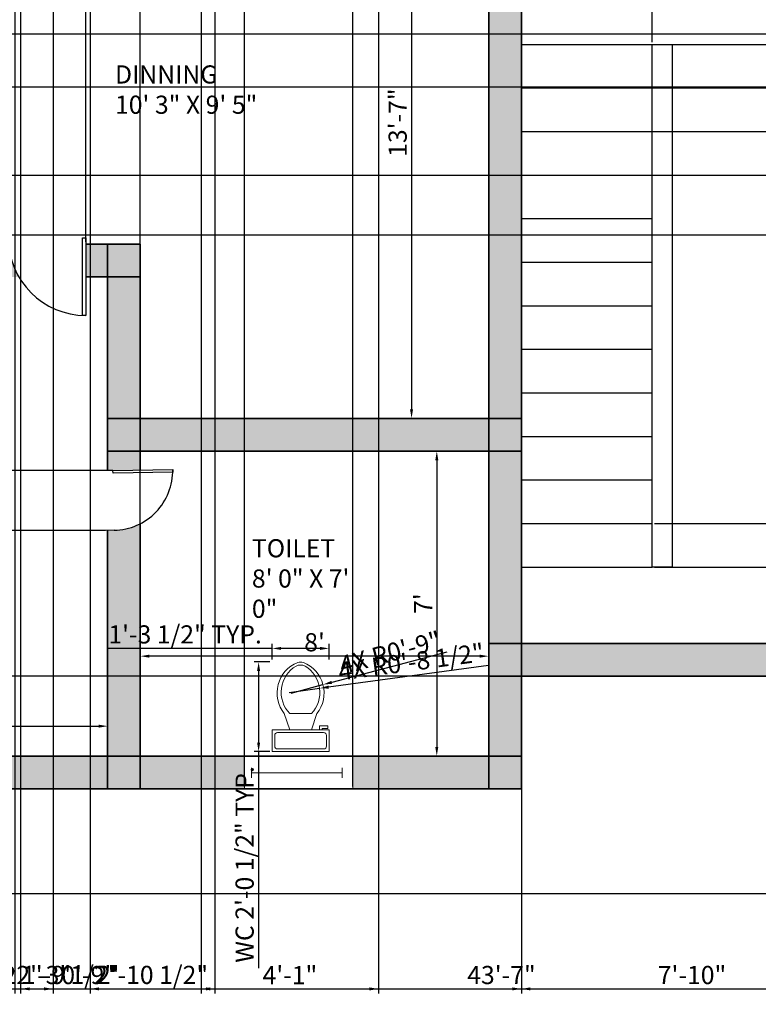
# Model space of a CAD drawing. Units: millimetres. Extents: x 2803 to 3393, y 965 to 1464.
# Tile 2 of 6: x 2968 to 3172, y 965 to 1236. Entities that reach past the tile are written whole.
import ezdxf

# ---------------------------------------------------------------- set-up
doc = ezdxf.new("R2010")
doc.units = ezdxf.units.MM
for name, color, linetype, lineweight in [('A-ANNO-DIMS', 150, 'Continuous', 18), ('A-AREA-IDEN', 200, 'Continuous', 25), ('A-FLOR-FIXT', 70, 'Continuous', 18), ('A-WALL-PATT', 2, 'Continuous', 13), ('doors', 10, 'Continuous', 25), ('staircase', 130, 'Continuous', 25), ('walls', 2, 'Continuous', 35), ('windows', 30, 'Continuous', 20)]:
    doc.layers.add(name, color=color, linetype=linetype, lineweight=lineweight)
doc.styles.get("Standard").update_dxf_attribs({"font": 'arial.ttf'})
doc.dimstyles.new('ISO-25', dxfattribs={"dimtxt": 5, "dimasz": 2.5, "dimexe": 1.25, "dimexo": 0.625, "dimtad": 1, "dimdec": 0, "dimlunit": 3, "dimtxsty": 'Standard', "dimcen": 2.5, "dimadec": 0, "dimazin": 0, "dimtfac": 1, "dimtdec": 0, "dimtmove": 0, "dimatfit": 3, "dimfxl": 1, "dimarcsym": 0})

# ---------------------------------------------------------------- blocks, each defined once
blk = doc.blocks.new('*U2')
for p, q in [((0, 0), (0, -6)), ((40, 0), (40, -6))]:
    blk.add_line(p, q)
blk.add_lwpolyline([(0, 0), (0, 40), (1.75, 40), (1.75, 0)], close=True)
blk.add_arc((0, 0), 40, 0, 90)
blk = doc.blocks.new('*U6')
for p, q in [((0, 4), (0, 0)), ((36, 4), (36, 0)), ((0, 2), (36, 2))]:
    blk.add_line(p, q)
blk = doc.blocks.new('Toilet - top')
for p, q in [((9.5, -6), (9.5, -2)), ((-10, -8.5), (-8, -8.5)), ((-10, -9.5), (-10, -8.5)), ((-7, -9.5), (-10, -9.5)), ((-8, -8.5), (-8, -8)), ((-7, -8), (-7, -9.5)), ((-4, -8), (-6, -14)), ((4, -8), (6, -14)), ((4, -14), (-4, -14))]:
    blk.add_line(p, q)
blk.add_lwpolyline([(10.5, -8), (10.5, 0), (-10.5, 0), (-10.5, -8)], close=True)
for points in [[(-9.5, -2), (-9.5, -6)], [(8.5, -1), (-8.5, -1)], [(-8.5, -7), (8.5, -7)]]:
    blk.add_lwpolyline(points)
for centre, radius, start, end in [((-8.62, -1.88), 0.884, 81.8699, 188.1301), ((8.62, -1.88), 0.884, 351.8699, 98.1301), ((-8.62, -6.12), 0.884, 171.8699, 278.1301), ((8.62, -6.12), 0.884, 261.8699, 8.1301), ((3.52, -21.58), 12.17, 141.4691, 247.9714), ((4.2, -21.82), 11.33, 136.3677, 238.9468), ((-3.52, -21.58), 12.17, 292.0284, 38.5307), ((-4.2, -21.82), 11.33, 301.053, 43.6321), ((0, -27.88), 4, 245.7318, 294.2682), ((0, -29), 4, 254.8605, 285.1395)]:
    blk.add_arc(centre, radius, start, end)
blk = doc.blocks.new('*D19')
at = {"layer": 'A-ANNO-DIMS', "color": 0, "lineweight": -2, "transparency": 16777216}
for p, q in [((3077.03, 1289.56), (3077.66, 1289.56)), ((3076.41, 1287.06), (3076.41, 1129.06)), ((3077.03, 1126.56), (3077.66, 1126.56))]:
    blk.add_line(p, q, dxfattribs=at)
at = {"layer": 'A-ANNO-DIMS', "color": 0, "transparency": 16777216}
for points in [[(3075.99, 1287.06), (3076.82, 1287.06), (3076.41, 1289.56)], [(3075.99, 1129.06), (3076.82, 1129.06), (3076.41, 1126.56)]]:
    blk.add_solid(points, dxfattribs=at)
at = {"layer": 'Defpoints', "color": 0, "transparency": 16777216}
for p in [(3076.41, 1289.56), (3076.41, 1126.56), (3076.41, 1126.56)]:
    blk.add_point(p, dxfattribs=at)
at = {"layer": 'A-ANNO-DIMS', "color": 0, "transparency": 16777216, "insert": (3073.23, 1208.06), "char_height": 5, "attachment_point": 5, "rotation": 90}
blk.add_mtext('13\'-7"', dxfattribs=at)
blk = doc.blocks.new('*D25')
at = {"layer": 'A-ANNO-DIMS', "color": 0, "lineweight": -2, "transparency": 16777216}
for p, q in [((2848.68, 1045.62), (2848.68, 1040.53)), ((2992.68, 1045.62), (2992.68, 1040.53)), ((2851.18, 1041.78), (2990.18, 1041.78))]:
    blk.add_line(p, q, dxfattribs=at)
at = {"layer": 'A-ANNO-DIMS', "color": 0, "transparency": 16777216}
for points in [[(2851.18, 1042.2), (2851.18, 1041.37), (2848.68, 1041.78)], [(2990.18, 1042.2), (2990.18, 1041.37), (2992.68, 1041.78)]]:
    blk.add_solid(points, dxfattribs=at)
at = {"layer": 'Defpoints', "color": 0, "transparency": 16777216}
for p in [(2848.68, 1046.25), (2992.68, 1046.25), (2992.68, 1041.78)]:
    blk.add_point(p, dxfattribs=at)
at = {"layer": 'A-ANNO-DIMS', "color": 0, "transparency": 16777216, "insert": (2920.68, 1044.92), "char_height": 5, "attachment_point": 5}
blk.add_mtext("12'", dxfattribs=at)
blk = doc.blocks.new('*D26')
at = {"layer": 'A-ANNO-DIMS', "color": 0, "lineweight": -2, "transparency": 16777216}
for p, q in [((3085.22, 1117.56), (3082.11, 1117.56)), ((3083.36, 1115.06), (3083.36, 1036.06)), ((3085.22, 1033.56), (3082.11, 1033.56))]:
    blk.add_line(p, q, dxfattribs=at)
at = {"layer": 'A-ANNO-DIMS', "color": 0, "transparency": 16777216}
for points in [[(3082.95, 1115.06), (3083.78, 1115.06), (3083.36, 1117.56)], [(3082.95, 1036.06), (3083.78, 1036.06), (3083.36, 1033.56)]]:
    blk.add_solid(points, dxfattribs=at)
at = {"layer": 'Defpoints', "color": 0, "transparency": 16777216}
for p in [(3085.85, 1117.56), (3083.36, 1033.56), (3085.85, 1033.56)]:
    blk.add_point(p, dxfattribs=at)
at = {"layer": 'A-ANNO-DIMS', "color": 0, "transparency": 16777216, "insert": (3080.24, 1075.56), "char_height": 5, "attachment_point": 5, "rotation": 90}
blk.add_mtext("7'", dxfattribs=at)
blk = doc.blocks.new('*D27')
at = {"layer": 'A-ANNO-DIMS', "color": 0, "lineweight": -2, "transparency": 16777216}
for p, q in [((3001.68, 1063.94), (3001.68, 1059.82)), ((3097.68, 1063.94), (3097.68, 1059.82)), ((3095.18, 1061.07), (3004.18, 1061.07))]:
    blk.add_line(p, q, dxfattribs=at)
at = {"layer": 'A-ANNO-DIMS', "color": 0, "transparency": 16777216}
for points in [[(3004.18, 1061.49), (3004.18, 1060.65), (3001.68, 1061.07)], [(3095.18, 1061.49), (3095.18, 1060.65), (3097.68, 1061.07)]]:
    blk.add_solid(points, dxfattribs=at)
at = {"layer": 'Defpoints', "color": 0, "transparency": 16777216}
for p in [(3001.68, 1064.56), (3097.68, 1064.56), (3001.68, 1061.07)]:
    blk.add_point(p, dxfattribs=at)
at = {"layer": 'A-ANNO-DIMS', "color": 0, "transparency": 16777216, "insert": (3049.68, 1064.25), "char_height": 5, "attachment_point": 5}
blk.add_mtext("8'", dxfattribs=at)
blk = doc.blocks.new('*D31')
at = {"layer": 'A-ANNO-DIMS', "color": 0, "lineweight": -2, "transparency": 16777216}
for p, q in [((3037.35, 1059.49), (3033.02, 1059.49)), ((3034.27, 1056.99), (3034.27, 1037.26)), ((3037.35, 1034.76), (3033.02, 1034.76)), ((3034.27, 1034.76), (3034.27, 975.1))]:
    blk.add_line(p, q, dxfattribs=at)
at = {"layer": 'A-ANNO-DIMS', "color": 0, "transparency": 16777216}
for points in [[(3033.85, 1056.99), (3034.68, 1056.99), (3034.27, 1059.49)], [(3033.85, 1037.26), (3034.68, 1037.26), (3034.27, 1034.76)]]:
    blk.add_solid(points, dxfattribs=at)
at = {"layer": 'Defpoints', "color": 0, "transparency": 16777216}
for p in [(3037.98, 1059.49), (3034.27, 1034.76), (3037.98, 1034.76)]:
    blk.add_point(p, dxfattribs=at)
at = {"layer": 'A-ANNO-DIMS', "color": 0, "transparency": 16777216, "insert": (3031.06, 1003.68), "char_height": 5, "attachment_point": 5, "rotation": 90}
blk.add_mtext('WC 2\'-0 1/2" TYP.', dxfattribs=at)
blk = doc.blocks.new('*D32')
at = {"layer": 'A-ANNO-DIMS', "color": 0, "lineweight": -2, "transparency": 16777216}
for p, q in [((3037.98, 1060.12), (3037.98, 1064.45)), ((3053.69, 1060.12), (3053.69, 1064.45)), ((3037.98, 1063.2), (2992.57, 1063.2)), ((3051.19, 1063.2), (3040.48, 1063.2))]:
    blk.add_line(p, q, dxfattribs=at)
at = {"layer": 'A-ANNO-DIMS', "color": 0, "transparency": 16777216}
for points in [[(3040.48, 1063.62), (3040.48, 1062.79), (3037.98, 1063.2)], [(3051.19, 1063.62), (3051.19, 1062.79), (3053.69, 1063.2)]]:
    blk.add_solid(points, dxfattribs=at)
at = {"layer": 'Defpoints', "color": 0, "transparency": 16777216}
for p in [(3037.98, 1063.2), (3037.98, 1059.49), (3053.69, 1059.49)]:
    blk.add_point(p, dxfattribs=at)
at = {"layer": 'A-ANNO-DIMS', "color": 0, "transparency": 16777216, "insert": (3014.02, 1066.42), "char_height": 5, "attachment_point": 5}
blk.add_mtext('1\'-3 1/2" TYP.', dxfattribs=at)
blk = doc.blocks.new('*D39')
at = {"layer": 'A-ANNO-DIMS', "color": 0, "lineweight": -2, "transparency": 16777216}
for p, q in [((2839.68, 1023.94), (2839.68, 968.15)), ((3362.68, 994.94), (3362.68, 968.15)), ((2842.18, 969.4), (3360.18, 969.4))]:
    blk.add_line(p, q, dxfattribs=at)
at = {"layer": 'A-ANNO-DIMS', "color": 0, "transparency": 16777216}
for points in [[(2842.18, 969.82), (2842.18, 968.99), (2839.68, 969.4)], [(3360.18, 969.82), (3360.18, 968.99), (3362.68, 969.4)]]:
    blk.add_solid(points, dxfattribs=at)
at = {"layer": 'Defpoints', "color": 0, "transparency": 16777216}
for p in [(2839.68, 1024.56), (3362.68, 995.56), (3362.68, 969.4)]:
    blk.add_point(p, dxfattribs=at)
at = {"layer": 'A-ANNO-DIMS', "color": 0, "transparency": 16777216, "insert": (3101.18, 972.58), "char_height": 5, "attachment_point": 5}
blk.add_mtext('43\'-7"', dxfattribs=at)
blk = doc.blocks.new('*D42')
at = {"layer": 'A-ANNO-DIMS', "color": 0, "lineweight": -2, "transparency": 16777216}
for p, q in [((3209.06, 1055.56), (2812.27, 1055.56)), ((2813.52, 998.06), (2813.52, 1053.06)), ((3209.06, 995.56), (2812.27, 995.56))]:
    blk.add_line(p, q, dxfattribs=at)
at = {"layer": 'A-ANNO-DIMS', "color": 0, "transparency": 16777216}
for points in [[(2813.11, 1053.06), (2813.94, 1053.06), (2813.52, 1055.56)], [(2813.11, 998.06), (2813.94, 998.06), (2813.52, 995.56)]]:
    blk.add_solid(points, dxfattribs=at)
at = {"layer": 'Defpoints', "color": 0, "transparency": 16777216}
for p in [(2813.52, 1055.56), (3209.68, 1055.56), (3209.68, 995.56)]:
    blk.add_point(p, dxfattribs=at)
at = {"layer": 'A-ANNO-DIMS', "color": 0, "transparency": 16777216, "insert": (2810.35, 1025.56), "char_height": 5, "attachment_point": 5, "rotation": 90}
blk.add_mtext('5\'-0"', dxfattribs=at)
blk = doc.blocks.new('*D43')
at = {"layer": 'A-ANNO-DIMS', "color": 0, "lineweight": -2, "transparency": 16777216}
for p, q in [((3106.68, 1230.24), (3106.68, 1454.97)), ((3142.68, 1230.24), (3142.68, 1454.97)), ((3109.18, 1453.72), (3140.18, 1453.72))]:
    blk.add_line(p, q, dxfattribs=at)
at = {"layer": 'A-ANNO-DIMS', "color": 0, "transparency": 16777216}
for points in [[(3109.18, 1454.14), (3109.18, 1453.31), (3106.68, 1453.72)], [(3140.18, 1454.14), (3140.18, 1453.31), (3142.68, 1453.72)]]:
    blk.add_solid(points, dxfattribs=at)
at = {"layer": 'Defpoints', "color": 0, "transparency": 16777216}
for p in [(3142.68, 1453.72), (3106.68, 1229.61), (3142.68, 1229.61)]:
    blk.add_point(p, dxfattribs=at)
at = {"layer": 'A-ANNO-DIMS', "color": 0, "transparency": 16777216, "insert": (3124.68, 1456.9), "char_height": 5, "attachment_point": 5}
blk.add_mtext('3\'-0"', dxfattribs=at)
blk = doc.blocks.new('*D44')
at = {"layer": 'A-ANNO-DIMS', "color": 0, "lineweight": -2, "transparency": 16777216}
for p, q in [((3148.87, 1229.61), (3390.09, 1229.61)), ((3388.84, 1088.11), (3388.84, 1227.11)), ((3148.87, 1085.61), (3390.09, 1085.61))]:
    blk.add_line(p, q, dxfattribs=at)
at = {"layer": 'A-ANNO-DIMS', "color": 0, "transparency": 16777216}
for points in [[(3388.43, 1227.11), (3389.26, 1227.11), (3388.84, 1229.61)], [(3388.43, 1088.11), (3389.26, 1088.11), (3388.84, 1085.61)]]:
    blk.add_solid(points, dxfattribs=at)
at = {"layer": 'Defpoints', "color": 0, "transparency": 16777216}
for p in [(3148.25, 1229.61), (3388.84, 1229.61), (3148.25, 1085.61)]:
    blk.add_point(p, dxfattribs=at)
at = {"layer": 'A-ANNO-DIMS', "color": 0, "transparency": 16777216, "insert": (3385.67, 1157.61), "char_height": 5, "attachment_point": 5, "rotation": 90}
blk.add_mtext('12\'-0"', dxfattribs=at)
blk = doc.blocks.new('*D45')
at = {"layer": 'A-ANNO-DIMS', "color": 0, "lineweight": -2, "transparency": 16777216}
for p, q in [((3200.68, 1297.94), (3200.68, 968.15)), ((3106.68, 1288.94), (3106.68, 968.15)), ((3109.18, 969.4), (3198.18, 969.4))]:
    blk.add_line(p, q, dxfattribs=at)
at = {"layer": 'A-ANNO-DIMS', "color": 0, "transparency": 16777216}
for points in [[(3109.18, 969.82), (3109.18, 968.99), (3106.68, 969.4)], [(3198.18, 969.82), (3198.18, 968.99), (3200.68, 969.4)]]:
    blk.add_solid(points, dxfattribs=at)
at = {"layer": 'Defpoints', "color": 0, "transparency": 16777216}
for p in [(3200.68, 1298.56), (3106.68, 1289.56), (3200.68, 969.4)]:
    blk.add_point(p, dxfattribs=at)
at = {"layer": 'A-ANNO-DIMS', "color": 0, "transparency": 16777216, "insert": (3153.68, 972.58), "char_height": 5, "attachment_point": 5}
blk.add_mtext('7\'-10"', dxfattribs=at)
blk = doc.blocks.new('*D46')
at = {"layer": 'A-ANNO-DIMS', "color": 0, "lineweight": -2, "transparency": 16777216}
for p, q in [((3067.93, 1289.56), (3390.09, 1289.56)), ((3388.84, 1232.11), (3388.84, 1287.06)), ((3201.31, 1229.61), (3390.09, 1229.61))]:
    blk.add_line(p, q, dxfattribs=at)
at = {"layer": 'A-ANNO-DIMS', "color": 0, "transparency": 16777216}
for points in [[(3388.43, 1287.06), (3389.26, 1287.06), (3388.84, 1289.56)], [(3388.43, 1232.11), (3389.26, 1232.11), (3388.84, 1229.61)]]:
    blk.add_solid(points, dxfattribs=at)
at = {"layer": 'Defpoints', "color": 0, "transparency": 16777216}
for p in [(3067.31, 1289.56), (3388.84, 1289.56), (3200.68, 1229.61)]:
    blk.add_point(p, dxfattribs=at)
at = {"layer": 'A-ANNO-DIMS', "color": 0, "transparency": 16777216, "insert": (3385.67, 1259.59), "char_height": 5, "attachment_point": 5, "rotation": 90}
blk.add_mtext('5\'-0"', dxfattribs=at)
blk = doc.blocks.new('*D47')
at = {"layer": 'A-ANNO-DIMS', "color": 0, "lineweight": -2, "transparency": 16777216}
for p, q in [((3388.84, 1097.61), (3388.84, 1114.18)), ((3143.31, 1097.61), (3390.09, 1097.61)), ((3388.84, 1088.11), (3388.84, 1095.11)), ((3143.31, 1085.61), (3390.09, 1085.61))]:
    blk.add_line(p, q, dxfattribs=at)
at = {"layer": 'A-ANNO-DIMS', "color": 0, "transparency": 16777216}
for points in [[(3388.43, 1095.11), (3389.26, 1095.11), (3388.84, 1097.61)], [(3388.43, 1088.11), (3389.26, 1088.11), (3388.84, 1085.61)]]:
    blk.add_solid(points, dxfattribs=at)
at = {"layer": 'Defpoints', "color": 0, "transparency": 16777216}
for p in [(3142.68, 1097.61), (3388.84, 1097.61), (3142.68, 1085.61)]:
    blk.add_point(p, dxfattribs=at)
at = {"layer": 'A-ANNO-DIMS', "color": 0, "transparency": 16777216, "insert": (3385.67, 1107.15), "char_height": 5, "attachment_point": 5, "rotation": 90}
blk.add_mtext('1\'-0"', dxfattribs=at)
blk = doc.blocks.new('*D48')
at = {"layer": 'A-ANNO-DIMS', "color": 0, "lineweight": -2, "transparency": 16777216}
for p, q in [((2839.68, 1023.94), (2839.68, 968.15)), ((3106.68, 1023.94), (3106.68, 968.15)), ((2842.18, 969.4), (3104.18, 969.4))]:
    blk.add_line(p, q, dxfattribs=at)
at = {"layer": 'A-ANNO-DIMS', "color": 0, "transparency": 16777216}
for points in [[(2842.18, 969.82), (2842.18, 968.99), (2839.68, 969.4)], [(3104.18, 969.82), (3104.18, 968.99), (3106.68, 969.4)]]:
    blk.add_solid(points, dxfattribs=at)
at = {"layer": 'Defpoints', "color": 0, "transparency": 16777216}
for p in [(2839.68, 1024.56), (3106.68, 1024.56), (3106.68, 969.4)]:
    blk.add_point(p, dxfattribs=at)
at = {"layer": 'A-ANNO-DIMS', "color": 0, "transparency": 16777216, "insert": (2973.18, 972.58), "char_height": 5, "attachment_point": 5}
blk.add_mtext('22\'-3"', dxfattribs=at)
blk = doc.blocks.new('*D61')
at = {"layer": 'A-ANNO-DIMS', "color": 0, "lineweight": -2, "transparency": 16777216}
for p, q in [((3001.68, 1025.19), (3001.68, 1454.97)), ((3030.4, 1025.19), (3030.4, 1454.97)), ((3004.18, 1453.72), (3027.9, 1453.72))]:
    blk.add_line(p, q, dxfattribs=at)
at = {"layer": 'A-ANNO-DIMS', "color": 0, "transparency": 16777216}
for points in [[(3004.18, 1454.14), (3004.18, 1453.31), (3001.68, 1453.72)], [(3027.9, 1454.14), (3027.9, 1453.31), (3030.4, 1453.72)]]:
    blk.add_solid(points, dxfattribs=at)
at = {"layer": 'Defpoints', "color": 0, "transparency": 16777216}
for p in [(3030.4, 1453.72), (3001.68, 1024.56), (3030.4, 1024.56)]:
    blk.add_point(p, dxfattribs=at)
at = {"layer": 'A-ANNO-DIMS', "color": 0, "transparency": 16777216, "insert": (3016.04, 1456.93), "char_height": 5, "attachment_point": 5}
blk.add_mtext('2\'-4 1/2"', dxfattribs=at)
blk = doc.blocks.new('*D62')
at = {"layer": 'A-ANNO-DIMS', "color": 0, "lineweight": -2, "transparency": 16777216}
for p, q in [((3030.4, 1025.19), (3030.4, 1454.97)), ((3060.2, 1025.19), (3060.2, 1454.97)), ((3032.9, 1453.72), (3057.7, 1453.72))]:
    blk.add_line(p, q, dxfattribs=at)
at = {"layer": 'A-ANNO-DIMS', "color": 0, "transparency": 16777216}
for points in [[(3032.9, 1454.14), (3032.9, 1453.31), (3030.4, 1453.72)], [(3057.7, 1454.14), (3057.7, 1453.31), (3060.2, 1453.72)]]:
    blk.add_solid(points, dxfattribs=at)
at = {"layer": 'Defpoints', "color": 0, "transparency": 16777216}
for p in [(3060.2, 1453.72), (3030.4, 1024.56), (3060.2, 1024.56)]:
    blk.add_point(p, dxfattribs=at)
at = {"layer": 'A-ANNO-DIMS', "color": 0, "transparency": 16777216, "insert": (3045.3, 1456.9), "char_height": 5, "attachment_point": 5}
blk.add_mtext('2\'-6"', dxfattribs=at)
blk = doc.blocks.new('*D63')
at = {"layer": 'A-ANNO-DIMS', "color": 0, "lineweight": -2, "transparency": 16777216}
for p, q in [((2968.68, 1426.94), (2968.68, 968.15)), ((2977.68, 1426.94), (2977.68, 968.15)), ((2971.18, 969.4), (2975.18, 969.4)), ((2977.68, 969.4), (2994.73, 969.4))]:
    blk.add_line(p, q, dxfattribs=at)
at = {"layer": 'A-ANNO-DIMS', "color": 0, "transparency": 16777216}
for points in [[(2971.18, 969.82), (2971.18, 968.99), (2968.68, 969.4)], [(2975.18, 969.82), (2975.18, 968.99), (2977.68, 969.4)]]:
    blk.add_solid(points, dxfattribs=at)
at = {"layer": 'Defpoints', "color": 0, "transparency": 16777216}
for p in [(2968.68, 1427.56), (2977.68, 1427.56), (2977.68, 969.4)]:
    blk.add_point(p, dxfattribs=at)
at = {"layer": 'A-ANNO-DIMS', "color": 0, "transparency": 16777216, "insert": (2987.45, 972.58), "char_height": 5, "attachment_point": 5}
blk.add_mtext('0\'-9"', dxfattribs=at)
blk = doc.blocks.new('*D64')
at = {"layer": 'A-ANNO-DIMS', "color": 0, "lineweight": -2, "transparency": 16777216}
for p, q in [((3018.47, 1288.94), (3018.47, 968.15)), ((3067.31, 1288.94), (3067.31, 968.15)), ((3020.97, 969.4), (3064.81, 969.4))]:
    blk.add_line(p, q, dxfattribs=at)
at = {"layer": 'A-ANNO-DIMS', "color": 0, "transparency": 16777216}
for points in [[(3020.97, 969.82), (3020.97, 968.99), (3018.47, 969.4)], [(3064.81, 969.82), (3064.81, 968.99), (3067.31, 969.4)]]:
    blk.add_solid(points, dxfattribs=at)
at = {"layer": 'Defpoints', "color": 0, "transparency": 16777216}
for p in [(3018.47, 1289.56), (3067.31, 1289.56), (3067.31, 969.4)]:
    blk.add_point(p, dxfattribs=at)
at = {"layer": 'A-ANNO-DIMS', "color": 0, "transparency": 16777216, "insert": (3042.89, 972.54), "char_height": 5, "attachment_point": 5}
blk.add_mtext('4\'-1"', dxfattribs=at)
blk = doc.blocks.new('*D65')
at = {"layer": 'A-ANNO-DIMS', "color": 0, "lineweight": -2, "transparency": 16777216}
for p, q in [((2987.84, 1244.19), (2987.84, 968.15)), ((3022.23, 1244.19), (3022.23, 968.15)), ((2990.34, 969.4), (3019.73, 969.4))]:
    blk.add_line(p, q, dxfattribs=at)
at = {"layer": 'A-ANNO-DIMS', "color": 0, "transparency": 16777216}
for points in [[(2990.34, 969.82), (2990.34, 968.99), (2987.84, 969.4)], [(3019.73, 969.82), (3019.73, 968.99), (3022.23, 969.4)]]:
    blk.add_solid(points, dxfattribs=at)
at = {"layer": 'Defpoints', "color": 0, "transparency": 16777216}
for p in [(2987.84, 1244.81), (3022.23, 1244.81), (3022.23, 969.4)]:
    blk.add_point(p, dxfattribs=at)
at = {"layer": 'A-ANNO-DIMS', "color": 0, "transparency": 16777216, "insert": (3005.03, 972.61), "char_height": 5, "attachment_point": 5}
blk.add_mtext('2\'-10 1/2"', dxfattribs=at)
blk = doc.blocks.new('*D67')
at = {"layer": 'A-ANNO-DIMS', "color": 0, "lineweight": -2, "transparency": 16777216}
for p, q in [((2945.75, 1288.94), (2945.75, 968.15)), ((2967.14, 1288.94), (2967.14, 968.15)), ((2948.25, 969.4), (2964.64, 969.4)), ((2967.14, 969.4), (2995.36, 969.4))]:
    blk.add_line(p, q, dxfattribs=at)
at = {"layer": 'A-ANNO-DIMS', "color": 0, "transparency": 16777216}
for points in [[(2948.25, 969.82), (2948.25, 968.99), (2945.75, 969.4)], [(2964.64, 969.82), (2964.64, 968.99), (2967.14, 969.4)]]:
    blk.add_solid(points, dxfattribs=at)
at = {"layer": 'Defpoints', "color": 0, "transparency": 16777216}
for p in [(2945.75, 1289.56), (2967.14, 1289.56), (2967.14, 969.4)]:
    blk.add_point(p, dxfattribs=at)
at = {"layer": 'A-ANNO-DIMS', "color": 0, "transparency": 16777216, "insert": (2982.5, 972.61), "char_height": 5, "attachment_point": 5}
blk.add_mtext('1\'-9 1/2"', dxfattribs=at)
blk = doc.blocks.new('*D69')
at = {"layer": 'A-ANNO-DIMS', "color": 0, "lineweight": -2, "transparency": 16777216}
for p, q in [((3388.84, 1193.62), (3388.84, 1221.84)), ((2942.31, 1193.62), (3390.09, 1193.62)), ((3388.84, 1179.64), (3388.84, 1191.12)), ((2942.31, 1177.14), (3390.09, 1177.14))]:
    blk.add_line(p, q, dxfattribs=at)
at = {"layer": 'A-ANNO-DIMS', "color": 0, "transparency": 16777216}
for points in [[(3388.43, 1191.12), (3389.26, 1191.12), (3388.84, 1193.62)], [(3388.43, 1179.64), (3389.26, 1179.64), (3388.84, 1177.14)]]:
    blk.add_solid(points, dxfattribs=at)
at = {"layer": 'Defpoints', "color": 0, "transparency": 16777216}
for p in [(2941.68, 1193.62), (3388.84, 1193.62), (2941.68, 1177.14)]:
    blk.add_point(p, dxfattribs=at)
at = {"layer": 'A-ANNO-DIMS', "color": 0, "transparency": 16777216, "insert": (3385.63, 1208.98), "char_height": 5, "attachment_point": 5, "rotation": 90}
blk.add_mtext('1\'-4 1/2"', dxfattribs=at)
blk = doc.blocks.new('*D70')
at = {"layer": 'A-ANNO-DIMS', "color": 0, "lineweight": -2, "transparency": 16777216}
for p, q in [((2965.38, 1175.19), (2965.38, 1454.97)), ((2986.69, 1175.19), (2986.69, 1454.97)), ((2967.88, 1453.72), (2984.19, 1453.72)), ((2986.69, 1453.72), (3014.92, 1453.72))]:
    blk.add_line(p, q, dxfattribs=at)
at = {"layer": 'A-ANNO-DIMS', "color": 0, "transparency": 16777216}
for points in [[(2967.88, 1454.14), (2967.88, 1453.31), (2965.38, 1453.72)], [(2984.19, 1454.14), (2984.19, 1453.31), (2986.69, 1453.72)]]:
    blk.add_solid(points, dxfattribs=at)
at = {"layer": 'Defpoints', "color": 0, "transparency": 16777216}
for p in [(2986.69, 1453.72), (2965.38, 1174.56), (2986.69, 1174.56)]:
    blk.add_point(p, dxfattribs=at)
at = {"layer": 'A-ANNO-DIMS', "color": 0, "transparency": 16777216, "insert": (3002.06, 1456.93), "char_height": 5, "attachment_point": 5}
blk.add_mtext('1\'-9 1/2"', dxfattribs=at)
blk = doc.blocks.new('*D71')
at = {"layer": 'A-ANNO-DIMS', "color": 0, "lineweight": -2, "transparency": 16777216}
for p, q in [((2813.52, 1112.21), (2813.52, 1140.43)), ((2992.06, 1112.21), (2812.27, 1112.21)), ((2813.52, 1098.23), (2813.52, 1109.71)), ((2992.06, 1095.73), (2812.27, 1095.73))]:
    blk.add_line(p, q, dxfattribs=at)
at = {"layer": 'A-ANNO-DIMS', "color": 0, "transparency": 16777216}
for points in [[(2813.11, 1109.71), (2813.94, 1109.71), (2813.52, 1112.21)], [(2813.11, 1098.23), (2813.94, 1098.23), (2813.52, 1095.73)]]:
    blk.add_solid(points, dxfattribs=at)
at = {"layer": 'Defpoints', "color": 0, "transparency": 16777216}
for p in [(2813.52, 1112.21), (2992.68, 1112.21), (2992.68, 1095.73)]:
    blk.add_point(p, dxfattribs=at)
at = {"layer": 'A-ANNO-DIMS', "color": 0, "transparency": 16777216, "insert": (2810.31, 1127.57), "char_height": 5, "attachment_point": 5, "rotation": 90}
blk.add_mtext('1\'-4 1/2"', dxfattribs=at)
blk = doc.blocks.new('*D74')
at = {"layer": 'A-ANNO-DIMS', "color": 0, "lineweight": -2, "transparency": 16777216}
for p, q in [((3388.84, 1232.56), (3388.84, 1260.78)), ((2869.11, 1232.56), (3390.09, 1232.56)), ((3388.84, 1220.39), (3388.84, 1230.06)), ((2933.31, 1217.89), (3390.09, 1217.89))]:
    blk.add_line(p, q, dxfattribs=at)
at = {"layer": 'A-ANNO-DIMS', "color": 0, "transparency": 16777216}
for points in [[(3388.43, 1230.06), (3389.26, 1230.06), (3388.84, 1232.56)], [(3388.43, 1220.39), (3389.26, 1220.39), (3388.84, 1217.89)]]:
    blk.add_solid(points, dxfattribs=at)
at = {"layer": 'Defpoints', "color": 0, "transparency": 16777216}
for p in [(2868.49, 1232.56), (3388.84, 1232.56), (2932.68, 1217.89)]:
    blk.add_point(p, dxfattribs=at)
at = {"layer": 'A-ANNO-DIMS', "color": 0, "transparency": 16777216, "insert": (3385.63, 1247.92), "char_height": 5, "attachment_point": 5, "rotation": 90}
blk.add_mtext('1\'-2 1/2"', dxfattribs=at)
blk = doc.blocks.new('*D79')
at = {"layer": 'A-ANNO-DIMS', "color": 0, "lineweight": -2, "transparency": 16777216}
for p, q in [((3086.12, 1062.19), (3054.43, 1053.86)), ((3043.2, 1050.91), (3052.01, 1053.23))]:
    blk.add_line(p, q, dxfattribs=at)
at = {"layer": 'A-ANNO-DIMS', "color": 0, "transparency": 16777216}
blk.add_solid([(3054.32, 1054.27), (3054.53, 1053.46), (3052.01, 1053.23)], dxfattribs=at)
at = {"layer": 'Defpoints', "color": 0, "transparency": 16777216}
for p in [(3052.01, 1053.23), (3043.2, 1050.91)]:
    blk.add_point(p, dxfattribs=at)
at = {"layer": 'A-ANNO-DIMS', "color": 0, "transparency": 16777216, "insert": (3070.68, 1061.42), "char_height": 5, "attachment_point": 5, "rotation": 14.7185}
blk.add_mtext('4X R0\'-9"', dxfattribs=at)
blk = doc.blocks.new('*D80')
at = {"layer": 'A-ANNO-DIMS', "color": 0, "lineweight": -2, "transparency": 16777216}
for p, q in [((3097.6, 1058.47), (3053.57, 1052.55)), ((3042.69, 1051.09), (3051.09, 1052.22))]:
    blk.add_line(p, q, dxfattribs=at)
at = {"layer": 'A-ANNO-DIMS', "color": 0, "transparency": 16777216}
blk.add_solid([(3053.52, 1052.97), (3053.63, 1052.14), (3051.09, 1052.22)], dxfattribs=at)
at = {"layer": 'Defpoints', "color": 0, "transparency": 16777216}
for p in [(3042.69, 1051.09), (3051.09, 1052.22)]:
    blk.add_point(p, dxfattribs=at)
at = {"layer": 'A-ANNO-DIMS', "color": 0, "transparency": 16777216, "insert": (3076.39, 1058.86), "char_height": 5, "attachment_point": 5, "rotation": 7.6565}
blk.add_mtext('4X R0\'-8 1/2"', dxfattribs=at)

msp = doc.modelspace()

# ---------------------------------------------------------------- hatches: boundary and pattern name
at = {"layer": 'A-WALL-PATT'}
h = msp.add_hatch(color=256, dxfattribs=at)
h.dxf.hatch_style = 1
h.paths.add_polyline_path([(2968.68, 1427.56), (2919.98, 1427.56), (2919.98, 1418.56), (2968.68, 1418.56)])
h.paths.add_polyline_path([(2977.68, 1427.56), (2968.68, 1427.56), (2968.68, 1418.56), (2977.68, 1418.56)])
h.paths.add_polyline_path([(2977.68, 1418.56), (2968.68, 1418.56), (2968.68, 1298.56), (2977.68, 1298.56)])
h.paths.add_polyline_path([(3021.74, 1427.56), (2977.68, 1427.56), (2977.68, 1418.56), (3021.74, 1418.56)])
h.paths.add_polyline_path([(2881.7, 1427.56), (2848.68, 1427.56), (2848.68, 1418.56), (2881.7, 1418.56)])
h.paths.add_polyline_path([(2848.68, 1427.56), (2839.68, 1427.56), (2839.68, 1418.56), (2848.68, 1418.56)])
h.paths.add_polyline_path([(2848.68, 1418.56), (2839.68, 1418.56), (2839.68, 1298.56), (2848.68, 1298.56)])
h.paths.add_polyline_path([(2932.68, 1298.56), (2848.68, 1298.56), (2848.68, 1289.56), (2932.68, 1289.56)])
h.paths.add_polyline_path([(2848.68, 1298.56), (2839.68, 1298.56), (2839.68, 1289.56), (2848.68, 1289.56)])
h.paths.add_polyline_path([(2848.68, 1289.56), (2839.68, 1289.56), (2839.68, 1280.88), (2848.68, 1280.88)])
h.paths.add_polyline_path([(2848.68, 1252.94), (2839.68, 1252.94), (2839.68, 1241.56), (2848.68, 1241.56)])
h.paths.add_polyline_path([(2848.68, 1241.56), (2839.68, 1241.56), (2839.68, 1232.56), (2848.68, 1232.56)])
h.paths.add_polyline_path([(2932.68, 1241.56), (2848.68, 1241.56), (2848.68, 1232.56), (2932.68, 1232.56)])
h.paths.add_polyline_path([(2941.68, 1241.56), (2932.68, 1241.56), (2932.68, 1232.56), (2941.68, 1232.56)])
h.paths.add_polyline_path([(2941.68, 1289.56), (2932.68, 1289.56), (2932.68, 1257.22, -0.114666), (2939.92, 1259.03), (2941.68, 1259.07)])
h.paths.add_polyline_path([(2941.68, 1298.56), (2932.68, 1298.56), (2932.68, 1289.56), (2941.68, 1289.56)])
h.paths.add_polyline_path([(2947.42, 1298.56), (2941.68, 1298.56), (2941.68, 1289.56), (2945.75, 1289.56), (2945.75, 1290.29, -0.099582)])
h.paths.add_polyline_path([(2977.68, 1298.56), (2968.68, 1298.56), (2968.68, 1289.56), (2977.68, 1289.56)])
h.paths.add_polyline_path([(3018.47, 1298.56), (2977.68, 1298.56), (2977.68, 1289.56), (3018.47, 1289.56)])
h.paths.add_polyline_path([(3097.68, 1298.56), (3067.31, 1298.56), (3067.31, 1289.56), (3097.68, 1289.56)])
h.paths.add_polyline_path([(3106.68, 1298.56), (3097.68, 1298.56), (3097.68, 1289.56), (3106.68, 1289.56)])
h.paths.add_polyline_path([(3200.68, 1298.56), (3106.68, 1298.56), (3106.68, 1289.56), (3200.68, 1289.56)])
h.paths.add_polyline_path([(3209.68, 1298.56), (3200.68, 1298.56), (3200.68, 1289.56), (3209.68, 1289.56)])
h.paths.add_polyline_path([(3209.68, 1289.56), (3200.68, 1289.56), (3200.68, 1270.22), (3209.68, 1270.22)])
h.paths.add_polyline_path([(3106.68, 1418.56), (3097.68, 1418.56), (3097.68, 1298.56), (3106.68, 1298.56)])
h.paths.add_polyline_path([(3106.68, 1427.56), (3097.68, 1427.56), (3097.68, 1418.56), (3106.68, 1418.56)])
h.paths.add_polyline_path([(3097.68, 1427.56), (3058.94, 1427.56), (3058.94, 1418.56), (3097.68, 1418.56)])
h.paths.add_polyline_path([(3353.68, 1427.56), (3106.68, 1427.56), (3106.68, 1418.56), (3353.68, 1418.56)])
h.paths.add_polyline_path([(3362.68, 1427.56), (3353.68, 1427.56), (3353.68, 1418.56), (3362.68, 1418.56)])
h.paths.add_polyline_path([(3362.68, 1418.56), (3353.68, 1418.56), (3353.68, 1064.56), (3362.68, 1064.56)])
h.paths.add_polyline_path([(3362.68, 1064.56), (3353.68, 1064.56), (3353.68, 1055.56), (3362.68, 1055.56)])
h.paths.add_polyline_path([(3362.68, 1055.56), (3353.68, 1055.56), (3353.68, 995.56), (3362.68, 995.56)])
h.paths.add_polyline_path([(3353.68, 1064.56), (3209.68, 1064.56), (3209.68, 1055.56), (3353.68, 1055.56)])
h.paths.add_polyline_path([(3200.68, 1064.56), (3106.68, 1064.56), (3106.68, 1055.56), (3200.68, 1055.56)])
h.paths.add_polyline_path([(3209.68, 1064.56), (3200.68, 1064.56), (3200.68, 1055.56), (3209.68, 1055.56)])
h.paths.add_polyline_path([(3209.68, 1229.61), (3200.68, 1229.61), (3200.68, 1064.56), (3209.68, 1064.56)])
h.paths.add_polyline_path([(3106.68, 1117.56), (3097.68, 1117.56), (3097.68, 1064.56), (3106.68, 1064.56)])
h.paths.add_polyline_path([(3106.68, 1126.56), (3097.68, 1126.56), (3097.68, 1117.56), (3106.68, 1117.56)])
h.paths.add_polyline_path([(3097.68, 1126.56), (3001.68, 1126.56), (3001.68, 1117.56), (3097.68, 1117.56)])
h.paths.add_polyline_path([(3001.68, 1165.56), (2992.68, 1165.56), (2992.68, 1126.56), (3001.68, 1126.56)])
h.paths.add_polyline_path([(3001.68, 1174.56), (2992.68, 1174.56), (2992.68, 1165.56), (3001.68, 1165.56)])
h.paths.add_polyline_path([(2992.68, 1174.56), (2986.69, 1174.56), (2986.69, 1165.56), (2992.68, 1165.56)])
h.paths.add_polyline_path([(3001.68, 1126.56), (2992.68, 1126.56), (2992.68, 1117.56), (3001.68, 1117.56)])
h.paths.add_polyline_path([(3001.68, 1117.56), (2992.68, 1117.56), (2992.68, 1112.21), (2994.15, 1112.23), (3001.68, 1112.37)])
h.paths.add_polyline_path([(3001.68, 1033.56), (2992.68, 1033.56), (2992.68, 1024.56), (3001.68, 1024.56)])
h.paths.add_polyline_path([(3001.68, 1097.58, -0.114732), (2994.45, 1095.76), (2992.68, 1095.73), (2992.68, 1033.56), (3001.68, 1033.56)])
h.paths.add_polyline_path([(3030.4, 1033.56), (3001.68, 1033.56), (3001.68, 1024.56), (3030.4, 1024.56)])
h.paths.add_polyline_path([(3097.68, 1033.56), (3060.2, 1033.56), (3060.2, 1024.56), (3097.68, 1024.56)])
h.paths.add_polyline_path([(3106.68, 1033.56), (3097.68, 1033.56), (3097.68, 1024.56), (3106.68, 1024.56)])
h.paths.add_polyline_path([(3106.68, 1055.56), (3097.68, 1055.56), (3097.68, 1033.56), (3106.68, 1033.56)])
h.paths.add_polyline_path([(3106.68, 1064.56), (3097.68, 1064.56), (3097.68, 1055.56), (3106.68, 1055.56)])
h.paths.add_polyline_path([(2992.68, 1033.56), (2848.68, 1033.56), (2848.68, 1024.56), (2992.68, 1024.56)])
h.paths.add_polyline_path([(2848.68, 1033.56), (2839.68, 1033.56), (2839.68, 1024.56), (2848.68, 1024.56)])
h.paths.add_polyline_path([(2848.68, 1070.54), (2839.68, 1070.54), (2839.68, 1033.56), (2848.68, 1033.56)])
h.paths.add_polyline_path([(2848.68, 1165.56), (2839.68, 1165.56), (2839.68, 1114.52), (2848.68, 1114.52)])
h.paths.add_polyline_path([(2848.68, 1174.56), (2839.68, 1174.56), (2839.68, 1165.56), (2848.68, 1165.56)])
h.paths.add_polyline_path([(2932.68, 1174.56), (2848.68, 1174.56), (2848.68, 1165.56), (2932.68, 1165.56)])
h.paths.add_polyline_path([(2941.68, 1174.56), (2932.68, 1174.56), (2932.68, 1165.56), (2941.68, 1165.56)])
h.paths.add_polyline_path([(2965.38, 1174.56), (2941.68, 1174.56), (2941.68, 1165.56), (2968.2, 1165.56, -0.111634)])
h.paths.add_polyline_path([(2848.68, 1193.13), (2839.68, 1193.13), (2839.68, 1174.56), (2848.68, 1174.56)])
h.paths.add_polyline_path([(2848.68, 1232.56), (2839.68, 1232.56), (2839.68, 1221.86), (2848.68, 1221.86)])
h.paths.add_polyline_path([(2941.68, 1232.56), (2932.68, 1232.56), (2932.68, 1191.24, -0.132111), (2940.91, 1193.6), (2941.68, 1193.62)])
h.paths.add_polyline_path([(3106.68, 1262.96), (3105.94, 1262.96, -0.099353), (3097.68, 1264.61), (3097.68, 1126.56), (3106.68, 1126.56)])

# ---------------------------------------------------------------- linework, layer by layer
at = {"layer": 'staircase'}
for p, q in [((3106.68, 1229.61), (3200.68, 1229.61)), ((3106.68, 1217.61), (3200.68, 1217.61)), ((3106.68, 1205.61), (3200.68, 1205.61)), ((3106.68, 1193.61), (3200.68, 1193.61)), ((3106.68, 1181.61), (3142.68, 1181.61)), ((3106.68, 1169.61), (3142.68, 1169.61)), ((3106.68, 1157.61), (3142.68, 1157.61)), ((3106.68, 1145.61), (3142.68, 1145.61)), ((3106.68, 1133.61), (3142.68, 1133.61)), ((3106.68, 1121.61), (3142.68, 1121.61)), ((3106.68, 1109.61), (3142.68, 1109.61)), ((3106.68, 1097.61), (3142.68, 1097.61)), ((3106.68, 1085.61), (3142.68, 1085.61))]:
    msp.add_line(p, q, dxfattribs=at)
msp.add_lwpolyline([(3142.68, 1229.61), (3148.25, 1229.61), (3148.25, 1085.61), (3142.68, 1085.61)], close=True, dxfattribs=at)
at = {"layer": 'walls'}
for p, q in [((3097.68, 1264.61), (3097.68, 1024.56)), ((3106.68, 1262.96), (3106.68, 1024.56)), ((2986.69, 1174.56), (3001.68, 1174.56)), ((2992.68, 1174.56), (2992.68, 1112.21)), ((3001.68, 1174.56), (3001.68, 1112.37)), ((2986.69, 1165.56), (3001.68, 1165.56)), ((3106.68, 1162.49), (3106.68, 1162.49)), ((2992.68, 1126.56), (3106.68, 1126.56)), ((2992.68, 1117.56), (3106.68, 1117.56)), ((3001.68, 1097.58), (3001.68, 1024.56)), ((2992.68, 1095.73), (2992.68, 1024.56)), ((3097.68, 1064.56), (3362.68, 1064.56)), ((3097.68, 1055.56), (3362.68, 1055.56)), ((2839.68, 1033.56), (3106.68, 1033.56)), ((2839.68, 1024.56), (3106.68, 1024.56))]:
    msp.add_line(p, q, dxfattribs=at)
at = {"layer": 'windows'}
for p, q in [((3030.4, 1033.56), (3030.4, 1024.56)), ((3060.2, 1033.56), (3060.2, 1024.56))]:
    msp.add_line(p, q, dxfattribs=at)

# ---------------------------------------------------------------- block references
at = {"layer": 'A-FLOR-FIXT', "xscale": 0.7483515901231887, "yscale": 0.7483515901231887, "zscale": 0.7483515901231887, "rotation": 180}
msp.add_blockref('Toilet - top', (3045.83, 1034.76), dxfattribs=at)
at = {"layer": 'doors'}
for p, xscale, yscale, zscale, rotation in [((2986.69, 1176.32), 0.534749261424752, 0.534749261424752, 0.534749261424752, 180), ((2994.15, 1112.23), 0.4118610338034785, 0.4118610338034785, 0.4118610338034785, 271.0241473025472)]:
    msp.add_blockref('*U2', p, dxfattribs=dict(at, xscale=xscale, yscale=yscale, zscale=zscale, rotation=rotation))
at = {"layer": 'windows', "xscale": 0.6948136988430634, "yscale": 0.6948136988430634, "zscale": 0.6948136988430634, "rotation": 180}
msp.add_blockref('*U6', (3057.3, 1030.32), dxfattribs=at)

# ---------------------------------------------------------------- texts
at = {"layer": 'A-AREA-IDEN', "char_height": 5, "attachment_point": 1}
for s, width, insert in [('DINNING \\P10\' 3" X 9\' 5"', 53.2067, (2994.71, 1223.83)), ('TOILET \\P8\' 0" X 7\' 0"', 34.1372, (3032.42, 1093.3))]:
    msp.add_mtext_dynamic_manual_height_columns(s, width=width, gutter_width=12.5, heights=[0], dxfattribs=dict(at, insert=insert))

# ---------------------------------------------------------------- dimensions: what is measured, and where the dimension line sits
at = {"layer": 'A-ANNO-DIMS'}
for base, p1, p2, override, picture, middle in [((2986.69, 1453.72), (2965.38, 1174.56), (2986.69, 1174.56), {"dimdec": 1, "dimlfac": 1, "dimrnd": 0, "dimzin": 1, "dimdsep": 46, "dimlunit": 4, "dimfrac": 2}, '*D70', (3002.06, 1456.93)), ((3030.4, 1453.72), (3001.68, 1024.56), (3030.4, 1024.56), {"dimdec": 1, "dimlfac": 1, "dimrnd": 0, "dimzin": 1, "dimdsep": 46, "dimlunit": 4, "dimfrac": 2}, '*D61', (3016.04, 1456.93)), ((3060.2, 1453.72), (3030.4, 1024.56), (3060.2, 1024.56), {"dimdec": 1, "dimlfac": 1, "dimrnd": 0, "dimzin": 1, "dimdsep": 46, "dimlunit": 4, "dimfrac": 2}, '*D62', (3045.3, 1456.9)), ((3142.68, 1453.72), (3106.68, 1229.61), (3142.68, 1229.61), {"dimdec": 1, "dimlfac": 1, "dimrnd": 0, "dimzin": 1, "dimdsep": 46, "dimlunit": 4, "dimfrac": 2}, '*D43', (3124.68, 1456.9)), ((2977.68, 969.4), (2968.68, 1427.56), (2977.68, 1427.56), {"dimdec": 1, "dimlfac": 1, "dimrnd": 0, "dimzin": 1, "dimdsep": 46, "dimlunit": 4, "dimfrac": 2}, '*D63', (2987.45, 972.58)), ((3200.68, 969.4), (3106.68, 1289.56), (3200.68, 1298.56), {"dimdec": 1, "dimlfac": 1, "dimrnd": 0, "dimzin": 1, "dimdsep": 46, "dimlunit": 4, "dimfrac": 2}, '*D45', (3153.68, 972.58)), ((2967.14, 969.4), (2945.75, 1289.56), (2967.14, 1289.56), {"dimdec": 1, "dimlfac": 1, "dimrnd": 0, "dimzin": 1, "dimdsep": 46, "dimlunit": 4, "dimfrac": 2}, '*D67', (2982.5, 972.61)), ((3067.31, 969.4), (3018.47, 1289.56), (3067.31, 1289.56), {"dimdec": 1, "dimlfac": 1, "dimrnd": 0, "dimzin": 1, "dimdsep": 46, "dimlunit": 4, "dimfrac": 2}, '*D64', (3042.89, 972.54)), ((3022.23, 969.4), (2987.84, 1244.81), (3022.23, 1244.81), {"dimdec": 1, "dimlfac": 1, "dimrnd": 0, "dimzin": 1, "dimdsep": 46, "dimlunit": 4, "dimfrac": 2}, '*D65', (3005.03, 972.61)), ((3001.68, 1061.07), (3097.68, 1064.56), (3001.68, 1064.56), {"dimclrd": 0, "dimclre": 0, "dimclrt": 0}, '*D27', (3049.68, 1064.25)), ((2992.68, 1041.78), (2848.68, 1046.25), (2992.68, 1046.25), {"dimclrd": 0, "dimclre": 0, "dimclrt": 0}, '*D25', (2920.68, 1044.92)), ((3362.68, 969.4), (2839.68, 1024.56), (3362.68, 995.56), {"dimdec": 1, "dimlfac": 1, "dimrnd": 0, "dimzin": 1, "dimdsep": 46, "dimlunit": 4, "dimfrac": 2}, '*D39', (3101.18, 972.58)), ((3106.68, 969.4), (2839.68, 1024.56), (3106.68, 1024.56), {"dimdec": 1, "dimlfac": 1, "dimrnd": 0, "dimzin": 1, "dimdsep": 46, "dimlunit": 4, "dimfrac": 2}, '*D48', (2973.18, 972.58))]:
    dim = msp.add_linear_dim(base=base, p1=p1, p2=p2, dimstyle='ISO-25', override=override, dxfattribs=at)
    dim.commit()
    dim.dimension.update_dxf_attribs({"geometry": picture, "text_midpoint": middle})
for base, p1, p2, override, picture, middle in [((3388.8438, 1289.563), (3200.6838, 1229.614), (3067.3091, 1289.563), {"dimdec": 1, "dimlfac": 1, "dimrnd": 0, "dimzin": 1, "dimdsep": 46, "dimlunit": 4, "dimfrac": 2}, '*D46', (3385.6659, 1259.5885)), ((3076.41, 1126.56), (3076.41, 1289.56), (3076.41, 1126.56), {"dimclrd": 0, "dimclre": 0, "dimclrt": 0}, '*D19', (3073.23, 1208.06)), ((3388.84, 1232.56), (2932.68, 1217.89), (2868.49, 1232.56), {"dimdec": 1, "dimlfac": 1, "dimrnd": 0, "dimzin": 1, "dimdsep": 46, "dimlunit": 4, "dimfrac": 2}, '*D74', (3385.63, 1247.92)), ((3388.84, 1229.61), (3148.25, 1085.61), (3148.25, 1229.61), {"dimdec": 1, "dimlfac": 1, "dimrnd": 0, "dimzin": 1, "dimdsep": 46, "dimlunit": 4, "dimfrac": 2}, '*D44', (3385.67, 1157.61)), ((3388.84, 1193.62), (2941.68, 1177.14), (2941.68, 1193.62), {"dimdec": 1, "dimlfac": 1, "dimrnd": 0, "dimzin": 1, "dimdsep": 46, "dimlunit": 4, "dimfrac": 2}, '*D69', (3385.63, 1208.98)), ((2813.52, 1112.21), (2992.68, 1095.73), (2992.68, 1112.21), {"dimdec": 1, "dimlfac": 1, "dimrnd": 0, "dimzin": 1, "dimdsep": 46, "dimlunit": 4, "dimfrac": 2}, '*D71', (2810.31, 1127.57)), ((3083.36, 1033.56), (3085.85, 1117.56), (3085.85, 1033.56), {"dimclrd": 0, "dimclre": 0, "dimclrt": 0}, '*D26', (3080.24, 1075.56)), ((3388.84, 1097.61), (3142.68, 1085.61), (3142.68, 1097.61), {"dimdec": 1, "dimlfac": 1, "dimrnd": 0, "dimzin": 1, "dimdsep": 46, "dimlunit": 4, "dimfrac": 2}, '*D47', (3385.67, 1107.15)), ((2813.52, 1055.56), (3209.68, 995.56), (3209.68, 1055.56), {"dimdec": 1, "dimlfac": 1, "dimrnd": 0, "dimzin": 1, "dimdsep": 46, "dimlunit": 4, "dimfrac": 2}, '*D42', (2810.35, 1025.56))]:
    dim = msp.add_linear_dim(base=base, p1=p1, p2=p2, angle=90, dimstyle='ISO-25', override=override, dxfattribs=at)
    dim.commit()
    dim.dimension.update_dxf_attribs({"geometry": picture, "text_midpoint": middle})
for base, p1, p2, angle, text, picture, middle in [((3037.98, 1063.2), (3053.69, 1059.49), (3037.98, 1059.49), 180, '<> TYP.', '*D32', (3014.02, 1066.42)), ((3034.27, 1034.76), (3037.98, 1059.49), (3037.98, 1034.76), 270, 'WC <> TYP.', '*D31', (3031.06, 1003.68))]:
    dim = msp.add_linear_dim(base=base, p1=p1, p2=p2, angle=angle, text=text, dimstyle='ISO-25', override={"dimdec": 1, "dimlfac": 1, "dimrnd": 0, "dimzin": 1, "dimdsep": 46, "dimlunit": 4, "dimfrac": 2}, dxfattribs=at)
    dim.commit()
    dim.dimension.update_dxf_attribs({"geometry": picture, "text_midpoint": middle})
for center, mpoint, picture, middle in [((3042.69, 1051.09), (3051.09, 1052.22), '*D80', (3076.39, 1058.86)), ((3043.2, 1050.91), (3052.01, 1053.23), '*D79', (3070.68, 1061.42))]:
    dim = msp.add_radius_dim(center=center, mpoint=mpoint, text='4X <>', dimstyle='ISO-25', override={"dimdec": 1, "dimlfac": 1, "dimrnd": 0, "dimzin": 1, "dimdsep": 46, "dimlunit": 4, "dimfrac": 2}, dxfattribs=at)
    dim.commit()
    dim.dimension.update_dxf_attribs({"geometry": picture, "text_midpoint": middle})

doc.saveas('drawing.dxf')
